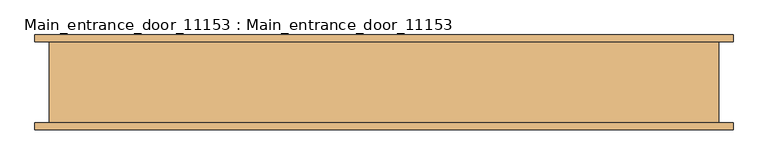
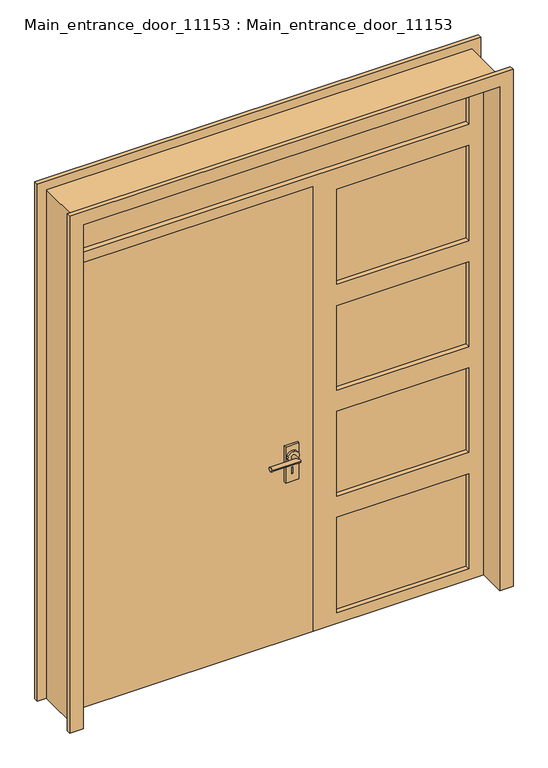
"""IFC4 building model written with IfcOpenShell, lengths in millimetres: door geometry, Main_entrance_door_11153 : Main_entrance_door_11153."""

from ifc_helpers import new_model, si_unit, point, frame, frame_2d, origin, origin_with_axes, place, context, project, spatial, polyline, circle_curve, ellipse_curve, trimmed, segment, composite_curve, outline, extrude, faceted_brep, source, transform, mapped, element, save
from ifc_brep_helpers import plane_surface, cylinder_surface, advanced_brep


def main_entrance_door_11153_main_entrance_door_11153_94c2f9e1(model_context):
    return source(origin(), model_context, "Body", "SolidModel", [
        advanced_brep(
        [(60.0, 60.0, 870.0), (80.0, 60.0, 870.0), (80.0, 100.0, 870.0), (60.0, 80.0, 870.0), (-50.0, 80.0, 870.0), (-50.0, 100.0, 870.0)],
        [
            (0, 1, circle_curve(frame((70.0, 60.0, 870.0), z_axis=(0.0, -1.0, 0.0), x_axis=(1.0, 0.0, 0.0)), 10.0)),
            (1, 0, circle_curve(frame((70.0, 60.0, 870.0), z_axis=(0.0, -1.0, 0.0), x_axis=(1.0, 0.0, 0.0)), 10.0)),
            (1, 2),
            (2, 3, ellipse_curve(frame((70.0, 90.0, 870.0), z_axis=(0.7071067811865411, -0.7071067811865538, 0.0), x_axis=(-0.7071067811865538, -0.7071067811865412, 0.0)), 14.1421356, 10.0)),
            (3, 0),
            (3, 2, ellipse_curve(frame((70.0, 90.0, 870.0), z_axis=(0.7071067811865411, -0.7071067811865538, 0.0), x_axis=(-0.7071067811865538, -0.7071067811865412, 0.0)), 14.1421356, 10.0)),
            (4, 5, circle_curve(frame((-50.0, 90.0, 870.0), z_axis=(-1.0, 0.0, 0.0), x_axis=(0.0, 1.0, 0.0)), 10.0)),
            (5, 4, circle_curve(frame((-50.0, 90.0, 870.0), z_axis=(-1.0, 0.0, 0.0), x_axis=(0.0, 1.0, 0.0)), 10.0)),
            (2, 5),
            (4, 3),
        ],
        [
            plane_surface(frame((70.0, 60.0, 870.0), z_axis=(0.0, -1.0, 0.0), x_axis=(0.0, 0.0, 1.0))),
            cylinder_surface(frame((70.0, 60.0, 870.0), z_axis=(0.0, -1.0, 0.0), x_axis=(1.0, 0.0, 0.0)), 10.0),
            plane_surface(frame((-50.0, 90.0, 870.0), z_axis=(-1.0, 0.0, 0.0), x_axis=(0.0, 0.0, 1.0))),
            cylinder_surface(frame((70.0, 90.0, 870.0), z_axis=(1.0, 0.0, 0.0), x_axis=(0.0, 1.0, 0.0)), 10.0),
        ],
        [
            (0, [[1, 2]]),
            (1, [[3, 4, 5, -2]]),
            (1, [[-5, 6, -3, -1]]),
            (2, [[7, 8]]),
            (3, [[9, -7, 10, -4]]),
            (3, [[-10, -8, -9, -6]]),
        ],
    ),
        extrude(outline(polyline([(920.0, 100.0), (920.0, 40.0), (750.0, 40.0), (750.0, 100.0), (920.0, 100.0)]), holes=[polyline([(815.3510082, 71.5671262), (785.3510082, 71.5671262), (785.3510082, 68.4328738), (815.3510082, 68.4328738), (815.3510082, 71.5671262)])]), frame((0.0, 40.0, 0.0), z_axis=(0.0, 1.0, 0.0), x_axis=(0.0, 0.0, 1.0)), (0.0, 0.0, 1.0), 10.0),
        extrude(outline(composite_curve([segment(trimmed(circle_curve(frame_2d((870.0, 70.0)), 25.0), [point((870.0, 45.0))], [point((870.0, 95.0))], False, "CARTESIAN"), True, "CONTINUOUS"), segment(trimmed(circle_curve(frame_2d((870.0, 70.0)), 25.0), [point((870.0, 95.0))], [point((870.0, 45.0))], False, "CARTESIAN"), True, "CONTINUOUS")], self_intersect=False)), frame((0.0, 40.0, 0.0), z_axis=(0.0, 1.0, 0.0), x_axis=(0.0, 0.0, 1.0)), (0.0, 0.0, 1.0), 20.0),
        advanced_brep(
        [(60.0, -30.0, 870.0), (80.0, -30.0, 870.0), (60.0, -50.0, 870.0), (80.0, -70.0, 870.0), (-50.0, -50.0, 870.0), (-50.0, -70.0, 870.0)],
        [
            (0, 1, circle_curve(frame((70.0, -30.0, 870.0), z_axis=(0.0, 1.0, 0.0), x_axis=(1.0, 0.0, 0.0)), 10.0)),
            (1, 0, circle_curve(frame((70.0, -30.0, 870.0), z_axis=(0.0, 1.0, 0.0), x_axis=(1.0, 0.0, 0.0)), 10.0)),
            (0, 2),
            (2, 3, ellipse_curve(frame((70.0, -60.0, 870.0), z_axis=(0.7071067811865457, 0.7071067811865492, 0.0), x_axis=(-0.7071067811865492, 0.7071067811865458, 0.0)), 14.1421356, 10.0)),
            (3, 1),
            (3, 2, ellipse_curve(frame((70.0, -60.0, 870.0), z_axis=(0.7071067811865457, 0.7071067811865492, 0.0), x_axis=(-0.7071067811865492, 0.7071067811865458, 0.0)), 14.1421356, 10.0)),
            (4, 5, circle_curve(frame((-50.0, -60.0, 870.0), z_axis=(-1.0, 0.0, 0.0), x_axis=(0.0, -1.0, 0.0)), 10.0)),
            (5, 4, circle_curve(frame((-50.0, -60.0, 870.0), z_axis=(-1.0, 0.0, 0.0), x_axis=(0.0, -1.0, 0.0)), 10.0)),
            (2, 4),
            (5, 3),
        ],
        [
            plane_surface(frame((70.0, -30.0, 870.0), z_axis=(0.0, 1.0, 0.0), x_axis=(0.0, 0.0, 1.0))),
            cylinder_surface(frame((70.0, -30.0, 870.0), z_axis=(0.0, 1.0, 0.0), x_axis=(1.0, 0.0, 0.0)), 10.0),
            plane_surface(frame((-50.0, -60.0, 870.0), z_axis=(-1.0, 0.0, 0.0), x_axis=(0.0, 0.0, 1.0))),
            cylinder_surface(frame((70.0, -60.0, 870.0), z_axis=(1.0, 0.0, 0.0), x_axis=(0.0, -1.0, 0.0)), 10.0),
        ],
        [
            (0, [[1, 2]]),
            (1, [[-1, 3, 4, 5]]),
            (1, [[-2, -5, 6, -3]]),
            (2, [[7, 8]]),
            (3, [[-4, 9, -8, 10]]),
            (3, [[-6, -10, -7, -9]]),
        ],
    ),
        extrude(outline(polyline([(920.0, 100.0), (920.0, 40.0), (750.0, 40.0), (750.0, 100.0), (920.0, 100.0)]), holes=[polyline([(815.3510082, 71.5671262), (785.3510082, 71.5671262), (785.3510082, 68.4328738), (815.3510082, 68.4328738), (815.3510082, 71.5671262)])]), frame((0.0, -20.0, 0.0), z_axis=(0.0, 1.0, 0.0), x_axis=(0.0, 0.0, 1.0)), (0.0, 0.0, 1.0), 10.0),
        extrude(outline(composite_curve([segment(trimmed(circle_curve(frame_2d((870.0, 70.0)), 25.0), [point((870.0, 45.0))], [point((870.0, 95.0))], False, "CARTESIAN"), True, "CONTINUOUS"), segment(trimmed(circle_curve(frame_2d((870.0, 70.0)), 25.0), [point((870.0, 95.0))], [point((870.0, 45.0))], False, "CARTESIAN"), True, "CONTINUOUS")], self_intersect=False)), frame((0.0, -30.0, 0.0), z_axis=(0.0, 1.0, 0.0), x_axis=(0.0, 0.0, 1.0)), (0.0, 0.0, 1.0), 20.0),
        faceted_brep([(990.0, 114.3, 0.0), (950.0, 114.3, 0.0), (950.0, -114.3, 0.0), (990.0, -114.3, 0.0), (990.0, -134.3, 0.0), (930.0, -134.3, 0.0), (930.0, 40.0, 0.0), (915.0, 40.0, 0.0), (915.0, 55.0, 0.0), (930.0, 55.0, 0.0), (930.0, 134.3, 0.0), (990.0, 134.3, 0.0), (990.0, 114.3, 2440.0), (-990.0, 114.3, 2440.0), (-990.0, 114.3, 0.0), (-950.0, 114.3, 0.0), (-950.0, 114.3, 2400.0), (950.0, 114.3, 2400.0), (950.0, -114.3, 2400.0), (-950.0, -114.3, 2400.0), (-950.0, -114.3, 0.0), (-990.0, -114.3, 0.0), (-990.0, -114.3, 2440.0), (990.0, -114.3, 2440.0), (990.0, -134.3, 2440.0), (-990.0, -134.3, 2440.0), (-990.0, -134.3, 0.0), (-930.0, -134.3, 0.0), (-930.0, -134.3, 2380.0), (930.0, -134.3, 2380.0), (930.0, 40.0, 2380.0), (-930.0, 40.0, 2380.0), (-930.0, 40.0, 0.0), (-915.0, 40.0, 0.0), (-915.0, 40.0, 2365.0), (915.0, 40.0, 2365.0), (915.0, 55.0, 2365.0), (-915.0, 55.0, 2365.0), (-915.0, 55.0, 0.0), (-930.0, 55.0, 0.0), (-930.0, 55.0, 2380.0), (930.0, 55.0, 2380.0), (930.0, 134.3, 2380.0), (-930.0, 134.3, 2380.0), (-930.0, 134.3, 0.0), (-990.0, 134.3, 0.0), (-990.0, 134.3, 2440.0), (990.0, 134.3, 2440.0)], [[[0, 1, 2, 3, 4, 5, 6, 7, 8, 9, 10, 11]], [[1, 0, 12, 13, 14, 15, 16, 17]], [[2, 1, 17, 18]], [[3, 2, 18, 19, 20, 21, 22, 23]], [[4, 3, 23, 24]], [[5, 4, 24, 25, 26, 27, 28, 29]], [[6, 5, 29, 30]], [[7, 6, 30, 31, 32, 33, 34, 35]], [[8, 7, 35, 36]], [[9, 8, 36, 37, 38, 39, 40, 41]], [[10, 9, 41, 42]], [[11, 10, 42, 43, 44, 45, 46, 47]], [[0, 11, 47, 12]], [[14, 13, 46, 45]], [[15, 14, 45, 44, 39, 38, 33, 32, 27, 26, 21, 20]], [[16, 15, 20, 19]], [[22, 21, 26, 25]], [[28, 27, 32, 31]], [[34, 33, 38, 37]], [[40, 39, 44, 43]], [[13, 12, 47, 46]], [[17, 16, 19, 18]], [[23, 22, 25, 24]], [[29, 28, 31, 30]], [[35, 34, 37, 36]], [[41, 40, 43, 42]]]),
        faceted_brep([(225.0, 40.0, 0.0), (930.0, 40.0, 0.0), (930.0, -10.0, 0.0), (170.0, -10.0, 0.0), (170.0, 40.0, 0.0), (155.0, 40.0, 0.0), (155.0, 55.0, 0.0), (225.0, 55.0, 0.0), (225.0, 40.0, 2100.0), (930.0, 40.0, 2100.0), (865.0, 40.0, 500.0), (275.0, 40.0, 500.0), (275.0, 40.0, 50.0), (865.0, 40.0, 50.0), (865.0, 40.0, 1000.0), (275.0, 40.0, 1000.0), (275.0, 40.0, 600.0), (865.0, 40.0, 600.0), (865.0, 40.0, 1500.0), (275.0, 40.0, 1500.0), (275.0, 40.0, 1100.0), (865.0, 40.0, 1100.0), (865.0, 40.0, 2050.0), (275.0, 40.0, 2050.0), (275.0, 40.0, 1600.0), (865.0, 40.0, 1600.0), (930.0, 55.0, 2100.0), (930.0, 55.0, 2380.0), (930.0, -10.0, 2380.0), (-930.0, -10.0, 2380.0), (-930.0, -10.0, 2100.0), (170.0, -10.0, 2100.0), (275.0, -10.0, 500.0), (865.0, -10.0, 500.0), (865.0, -10.0, 50.0), (275.0, -10.0, 50.0), (275.0, -10.0, 1000.0), (865.0, -10.0, 1000.0), (865.0, -10.0, 600.0), (275.0, -10.0, 600.0), (-880.0, -10.0, 2315.0), (865.0, -10.0, 2315.0), (865.0, -10.0, 2150.0), (-880.0, -10.0, 2150.0), (275.0, -10.0, 1500.0), (865.0, -10.0, 1500.0), (865.0, -10.0, 1100.0), (275.0, -10.0, 1100.0), (275.0, -10.0, 2050.0), (865.0, -10.0, 2050.0), (865.0, -10.0, 1600.0), (275.0, -10.0, 1600.0), (170.0, 40.0, 2100.0), (155.0, 40.0, 2100.0), (155.0, 55.0, 2100.0), (-930.0, 55.0, 2100.0), (-930.0, 55.0, 2380.0), (225.0, 55.0, 2100.0), (865.0, 55.0, 2315.0), (-880.0, 55.0, 2315.0), (-880.0, 55.0, 2150.0), (865.0, 55.0, 2150.0)], [[[0, 1, 2, 3, 4, 5, 6, 7]], [[1, 0, 8, 9], [10, 11, 12, 13], [14, 15, 16, 17], [18, 19, 20, 21], [22, 23, 24, 25]], [[2, 1, 9, 26, 27, 28]], [[3, 2, 28, 29, 30, 31], [32, 33, 34, 35], [36, 37, 38, 39], [40, 41, 42, 43], [44, 45, 46, 47], [48, 49, 50, 51]], [[4, 3, 31, 52]], [[5, 4, 52, 53]], [[6, 5, 53, 54]], [[7, 6, 54, 55, 56, 27, 26, 57], [58, 59, 60, 61]], [[0, 7, 57, 8]], [[10, 33, 32, 11]], [[33, 10, 13, 34]], [[12, 35, 34, 13]], [[11, 32, 35, 12]], [[14, 37, 36, 15]], [[37, 14, 17, 38]], [[16, 39, 38, 17]], [[15, 36, 39, 16]], [[45, 18, 21, 46]], [[20, 47, 46, 21]], [[19, 44, 47, 20]], [[27, 56, 29, 28]], [[29, 56, 55, 30]], [[58, 41, 40, 59]], [[41, 58, 61, 42]], [[59, 40, 43, 60]], [[18, 45, 44, 19]], [[22, 49, 48, 23]], [[24, 51, 50, 25]], [[23, 48, 51, 24]], [[49, 22, 25, 50]], [[57, 26, 9, 8]], [[30, 55, 54, 53, 52, 31]], [[60, 43, 42, 61]]]),
        extrude(outline(polyline([(170.0, 40.0), (170.0, -10.0), (-930.0, -10.0), (-930.0, 40.0), (170.0, 40.0)])), origin_with_axes(), (0.0, 0.0, 1.0), 2100.0),
        extrude(outline(polyline([(-880.0, 12.0), (-880.0, 18.0), (865.0, 18.0), (865.0, 12.0), (-880.0, 12.0)])), frame((0.0, 0.0, 2150.0), z_axis=(0.0, 0.0, 1.0), x_axis=(1.0, 0.0, 0.0)), (0.0, 0.0, 1.0), 165.0),
        extrude(outline(polyline([(865.0, 18.0), (865.0, 12.0), (275.0, 12.0), (275.0, 18.0), (865.0, 18.0)])), frame((0.0, 0.0, 50.0), z_axis=(0.0, 0.0, 1.0), x_axis=(1.0, 0.0, 0.0)), (0.0, 0.0, 1.0), 450.0),
        extrude(outline(polyline([(865.0, 18.0), (865.0, 12.0), (275.0, 12.0), (275.0, 18.0), (865.0, 18.0)])), frame((0.0, 0.0, 600.0), z_axis=(0.0, 0.0, 1.0), x_axis=(1.0, 0.0, 0.0)), (0.0, 0.0, 1.0), 400.0),
        extrude(outline(polyline([(865.0, 18.0), (865.0, 12.0), (275.0, 12.0), (275.0, 18.0), (865.0, 18.0)])), frame((0.0, 0.0, 1600.0), z_axis=(0.0, 0.0, 1.0), x_axis=(1.0, 0.0, 0.0)), (0.0, 0.0, 1.0), 450.0),
        extrude(outline(polyline([(865.0, 18.0), (865.0, 12.0), (275.0, 12.0), (275.0, 18.0), (865.0, 18.0)])), frame((0.0, 0.0, 1100.0), z_axis=(0.0, 0.0, 1.0), x_axis=(1.0, 0.0, 0.0)), (0.0, 0.0, 1.0), 400.0),
    ])


if __name__ == "__main__":
    model = new_model("IFC4")
    model_context = context("Model", 3, world=origin())
    ifc_project = project(units=[si_unit("LENGTHUNIT", "METRE", prefix="MILLI")], contexts=[model_context])
    site = spatial("IfcSite", under=ifc_project)
    building = spatial("IfcBuilding", under=site)
    placement = place(None, origin())
    main_entrance_door_11153_main_entrance_door_11153_shape = main_entrance_door_11153_main_entrance_door_11153_94c2f9e1(model_context)
    element("IfcDoor", 1, ObjectType="Main_entrance_door_11153 : Main_entrance_door_11153", at=placement, inside=building, context=model_context, shape_type="MappedRepresentation", body=[
        mapped(main_entrance_door_11153_main_entrance_door_11153_shape, transform((0.0, 0.0, 0.0), x_axis=(1.0, 0.0, 0.0), y_axis=(0.0, 1.0, 0.0), z_axis=(0.0, 0.0, 1.0))),
    ])
    save(model, "model.ifc")

# Revit data of these elements
# Type "Main_entrance_door_11153 : Main_entrance_door_11153"
#   Type Mark = "22"
#   Height = 7' - 10.48819"
#   Width = 6' - 2.80315"
#   Door Width = 3' - 7.30709"
#   Function = (empty or 0)
#   Wall Closure = (empty or 0)
# Element 1 (IfcDoor, "Main_entrance_door_11153 : Main_entrance_door_11153")
#   Materials on its faces: "Glass", "Default"
# Materials
#   "Glass": class "Glass", colour RGB 0 128 192, transparency 0.75, Description = "Soda Lime Glass", Cost = 0
#   "Default": colour RGB 127 127 127, transparency 0, Cost = 0
